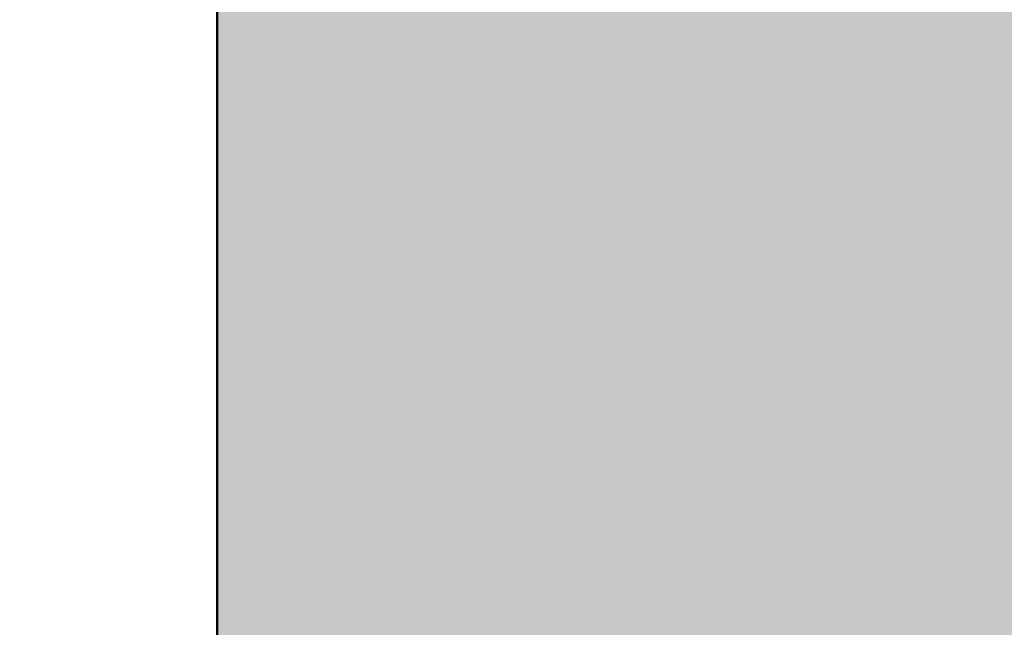
# Model space of a CAD drawing. Units: millimetres. Extents: x 0 to 2267, y 0 to 1823.
# Tile 32 of 256: x 1593.3409 to 1593.7801, y 1226.1145 to 1226.3857. Entities that reach past the tile are written whole.
import ezdxf

# ---------------------------------------------------------------- set-up
doc = ezdxf.new("R2010")
doc.units = ezdxf.units.MM
doc.header["$MEASUREMENT"] = 0
doc.layers.add('M-HATC', color=252, linetype='Continuous', lineweight=18)
doc.layers.add('M-OUTL', color=7, linetype='Continuous', lineweight=50)

msp = doc.modelspace()

# ---------------------------------------------------------------- hatches: boundary and pattern name
at = {"layer": 'M-HATC'}
h = msp.add_hatch(color=256, dxfattribs=at)
h.dxf.hatch_style = 1
h.paths.add_polyline_path([(2055.77105, 1603.06204), (1381.08677, 1603.06204), (1381.08677, 1598.06204), (2055.77105, 1598.06204)])
h.paths.add_polyline_path([(2055.77105, 1598.06204), (1381.08677, 1598.06204), (1381.08677, 1593.06204), (2055.77105, 1593.06204)])
h.paths.add_polyline_path([(2051.30737, 1536.76088), (1385.55044, 1536.76088), (1385.55044, 1526.76088), (1387.55044, 1526.76088), (1388.53662, 1525.05276), (1385.33187, 1521.23348), (1385.33187, 1521.22256), (2050.25417, 1522.74913), (2048.32119, 1525.05276), (2049.30737, 1526.76088), (2051.30737, 1526.76088)])
edge = h.paths.add_edge_path()
edge.add_arc((1847.53451, 1379.14917), 135, 222.6030607, 222.8908505, ccw=False)
edge.add_line((1748.16629, 1287.76561), (1683.09212, 1287.76561))
edge.add_arc((1583.7239, 1379.14917), 135, 317.1091495, 317.3969393, ccw=False)
edge.add_arc((1678.9686, 1290.67067), 5, 222.89085, 317.10915, ccw=False)
edge.add_arc((1774.21331, 1379.14917), 135, 222.6030607, 222.8908505, ccw=False)
edge.add_line((1674.84509, 1287.76561), (1609.77092, 1287.76561))
edge.add_arc((1510.4027, 1379.14917), 135, 317.1091495, 317.3969393, ccw=False)
edge.add_arc((1605.6474, 1290.67067), 5, 222.89085, 317.10915, ccw=False)
edge.add_arc((1700.89211, 1379.14917), 135, 222.6030607, 222.8908505, ccw=False)
edge.add_line((1601.52388, 1287.76561), (1536.44972, 1287.76561))
edge.add_arc((1437.08149, 1379.14917), 135, 317.1091495, 317.3969393, ccw=False)
edge.add_arc((1532.3262, 1290.67067), 5, 222.89085, 317.10915, ccw=False)
edge.add_arc((1627.57091, 1379.14917), 135, 222.6030607, 222.8908505, ccw=False)
edge.add_line((1528.20268, 1287.76561), (1505.92891, 1287.76561))
edge.add_spline(control_points=[(1505.92891, 1287.76561), (1504.26224, 1287.76561), (1504.26224, 1282.76561), (1505.92891, 1282.76561)], knot_values=[0, 0, 0, 0, 5, 5, 5, 5], degree=3, periodic=0)
edge.add_line((1505.92891, 1282.76561), (1930.92891, 1282.76561))
edge.add_spline(control_points=[(1930.92891, 1282.76561), (1932.59557, 1282.76561), (1932.59557, 1287.76561), (1930.92891, 1287.76561)], knot_values=[0, 0, 0, 0, 5, 5, 5, 5], degree=3, periodic=0)
edge.add_line((1930.92891, 1287.76561), (1903.05573, 1287.76561))
edge.add_arc((1803.6875, 1379.14917), 135, 317.1091495, 317.3969393, ccw=False)
edge.add_arc((1898.93221, 1290.67067), 5, 222.89085, 317.10915, ccw=False)
edge.add_arc((1994.17691, 1379.14917), 135, 222.6030607, 222.8908505, ccw=False)
edge.add_line((1894.80869, 1287.76561), (1829.73452, 1287.76561))
edge.add_arc((1730.3663, 1379.14917), 135, 317.1091495, 317.3969393, ccw=False)
edge.add_arc((1825.61101, 1290.67067), 5, 222.89085, 317.10915, ccw=False)
edge.add_arc((1920.85571, 1379.14917), 135, 222.6030607, 222.8908505, ccw=False)
edge.add_line((1821.48749, 1287.76561), (1756.41332, 1287.76561))
edge.add_arc((1657.0451, 1379.14917), 135, 317.1091495, 317.3969393, ccw=False)
edge.add_arc((1752.28981, 1290.67067), 5, 222.89085, 317.10915, ccw=False)
edge = h.paths.add_edge_path()
edge.add_spline(control_points=[(1843.42891, 1227.24746), (1845.09557, 1227.24746), (1845.09557, 1232.24746), (1843.42891, 1232.24746)], knot_values=[0, 0, 0, 0, 5, 5, 5, 5], degree=3, periodic=0)
edge.add_line((1843.42891, 1232.24746), (1593.42891, 1232.24746))
edge.add_spline(control_points=[(1593.42891, 1232.24746), (1591.76224, 1232.24746), (1591.76224, 1227.24746), (1593.42891, 1227.24746)], knot_values=[0, 0, 0, 0, 5, 5, 5, 5], degree=3, periodic=0)
edge.add_line((1593.42891, 1227.24746), (1843.42891, 1227.24746))
h.paths.add_polyline_path([(1905.92891, 1127.41706), (1530.92891, 1127.41706, 0.414214), (1520.92891, 1117.41706), (1530.92891, 1117.41706), (1915.92891, 1117.41706, 0.414214)])
edge = h.paths.add_edge_path()
edge.add_arc((1397.08577, 1498.40775), 12.72993, 90.782146, 190.878706, ccw=False)
edge.add_line((1396.912, 1511.13649), (1428.00968, 1511.34875))
edge.add_line((1428.00968, 1511.34875), (1433.00968, 1511.34875))
edge.add_line((1433.00968, 1511.34875), (1434.439, 1511.34875))
edge.add_arc((1419.474, 1498.08041), 20, 41.560995, 74.082109)
edge.add_line((1424.95919, 1517.31353), (1399.93509, 1517.25608))
edge.add_spline(control_points=[(1399.93074, 1517.25607), (1399.88398, 1517.21312), (1399.8328, 1517.16893), (1399.77741, 1517.1236)], knot_values=[11.567499, 11.567499, 11.567499, 11.567499, 11.814249, 11.814249, 11.814249, 11.814249], degree=3, periodic=0)
edge.add_spline(control_points=[(1399.63279, 1517.00986), (1399.58305, 1516.97214), (1399.53072, 1516.93375), (1399.47591, 1516.89474)], knot_values=[11.167718, 11.167718, 11.167718, 11.167718, 11.365188, 11.365188, 11.365188, 11.365188], degree=3, periodic=0)
edge.add_spline(control_points=[(1399.33981, 1516.80007), (1399.15144, 1516.67185), (1398.93836, 1516.5377), (1398.70404, 1516.39942)], knot_values=[10.376405, 10.376405, 10.376405, 10.376405, 11.00994, 11.00994, 11.00994, 11.00994], degree=3, periodic=0)
edge.add_spline(control_points=[(1398.65716, 1516.37187), (1398.57885, 1516.32602), (1398.49825, 1516.27974), (1398.41549, 1516.23309)], knot_values=[10.125175, 10.125175, 10.125175, 10.125175, 10.334406, 10.334406, 10.334406, 10.334406], degree=3, periodic=0)
edge.add_spline(control_points=[(1398.26422, 1516.14874), (1398.19595, 1516.11107), (1398.12634, 1516.07319), (1398.05546, 1516.03513)], knot_values=[9.832246, 9.832246, 9.832246, 9.832246, 9.999658, 9.999658, 9.999658, 9.999658], degree=3, periodic=0)
edge.add_spline(control_points=[(1397.9987, 1516.00476), (1397.73115, 1515.86211), (1397.44602, 1515.71707), (1397.14664, 1515.57138)], knot_values=[9.161808, 9.161808, 9.161808, 9.161808, 9.787769, 9.787769, 9.787769, 9.787769], degree=3, periodic=0)
edge.add_spline(control_points=[(1397.14664, 1515.57138), (1396.84182, 1515.42305), (1396.52223, 1515.27404), (1396.1914, 1515.12621)], knot_values=[8.524455, 8.524455, 8.524455, 8.524455, 9.161808, 9.161808, 9.161808, 9.161808], degree=3, periodic=0)
edge.add_spline(control_points=[(1396.07771, 1515.07565), (1395.98538, 1515.03478), (1395.89222, 1514.99402), (1395.7983, 1514.9534)], knot_values=[8.275193, 8.275193, 8.275193, 8.275193, 8.451726, 8.451726, 8.451726, 8.451726], degree=3, periodic=0)
edge.add_spline(control_points=[(1395.60184, 1514.86912), (1395.49975, 1514.82568), (1395.39685, 1514.78244), (1395.29322, 1514.73944)], knot_values=[7.962917, 7.962917, 7.962917, 7.962917, 8.152764, 8.152764, 8.152764, 8.152764], degree=3, periodic=0)
edge.add_spline(control_points=[(1395.21158, 1514.70568), (1394.82779, 1514.5475), (1394.43452, 1514.39287), (1394.03645, 1514.24422)], knot_values=[7.21254, 7.21254, 7.21254, 7.21254, 7.913148, 7.913148, 7.913148, 7.913148], degree=3, periodic=0)
edge.add_spline(control_points=[(1394.03645, 1514.24422), (1393.70758, 1514.12142), (1393.37544, 1514.0027), (1393.04267, 1513.88945)], knot_values=[6.633733, 6.633733, 6.633733, 6.633733, 7.21254, 7.21254, 7.21254, 7.21254], degree=3, periodic=0)
edge.add_spline(control_points=[(1392.82142, 1513.81499), (1392.71978, 1513.78118), (1392.61815, 1513.74791), (1392.51658, 1513.71521)], knot_values=[6.328796, 6.328796, 6.328796, 6.328796, 6.505493, 6.505493, 6.505493, 6.505493], degree=3, periodic=0)
edge.add_spline(control_points=[(1392.51658, 1513.71521), (1392.31873, 1513.65151), (1392.12116, 1513.59001), (1391.92441, 1513.53098)], knot_values=[5.984605, 5.984605, 5.984605, 5.984605, 6.328796, 6.328796, 6.328796, 6.328796], degree=3, periodic=0)
edge.add_spline(control_points=[(1391.79155, 1513.49146), (1391.31215, 1513.35011), (1390.83842, 1513.22392), (1390.37844, 1513.11711)], knot_values=[5.066697, 5.066697, 5.066697, 5.066697, 5.907055, 5.907055, 5.907055, 5.907055], degree=3, periodic=0)
edge.add_spline(control_points=[(1390.37844, 1513.11711), (1390.17973, 1513.07097), (1389.98359, 1513.02845), (1389.79067, 1512.98988)], knot_values=[4.70367, 4.70367, 4.70367, 4.70367, 5.066695, 5.066695, 5.066695, 5.066695], degree=3, periodic=0)
edge.add_spline(control_points=[(1389.42203, 1512.92036), (1389.24588, 1512.88922), (1389.0729, 1512.86172), (1388.90364, 1512.83814)], knot_values=[4.130571, 4.130571, 4.130571, 4.130571, 4.469816, 4.469816, 4.469816, 4.469816], degree=3, periodic=0)
edge.add_spline(control_points=[(1388.90364, 1512.83814), (1388.59103, 1512.7946), (1388.29108, 1512.76444), (1388.00714, 1512.74941)], knot_values=[3.504031, 3.504031, 3.504031, 3.504031, 4.130571, 4.130571, 4.130571, 4.130571], degree=3, periodic=0)
edge.add_spline(control_points=[(1387.9356, 1512.74593), (1387.85378, 1512.74231), (1387.77334, 1512.73997), (1387.69435, 1512.73898)], knot_values=[3.268866, 3.268866, 3.268866, 3.268866, 3.451164, 3.451164, 3.451164, 3.451164], degree=3, periodic=0)
edge.add_spline(control_points=[(1387.33512, 1512.74426), (1387.20757, 1512.74991), (1387.08472, 1512.7597), (1386.96699, 1512.77385)], knot_values=[2.670686, 2.670686, 2.670686, 2.670686, 2.984, 2.984, 2.984, 2.984], degree=3, periodic=0)
edge.add_spline(control_points=[(1386.83274, 1512.79225), (1386.82093, 1512.79407), (1386.80917, 1512.79594), (1386.79747, 1512.79787)], knot_values=[2.516981, 2.516981, 2.516981, 2.516981, 2.549528, 2.549528, 2.549528, 2.549528], degree=3, periodic=0)
edge.add_spline(control_points=[(1386.45257, 1512.87348), (1386.42573, 1512.88105), (1386.39931, 1512.88895), (1386.3733, 1512.89719)], knot_values=[2.095869, 2.095869, 2.095869, 2.095869, 2.17941, 2.17941, 2.17941, 2.17941], degree=3, periodic=0)
edge.add_spline(control_points=[(1386.06911, 1513.01889), (1386.06338, 1513.02174), (1386.05768, 1513.02463), (1386.05201, 1513.02753)], knot_values=[1.72453, 1.72453, 1.72453, 1.72453, 1.745933, 1.745933, 1.745933, 1.745933], degree=3, periodic=0)
edge.add_arc((1399.474, 1498.08041), 20, 131.824322, 180)
edge.add_arc((1630.33362, 1505.54843), 250.97076, 181.7051759, 236.427975)
edge.add_arc((1605.33992, 1483.30441), 218.7822, 238.660829, 243.3496099)
edge.add_arc((1647.09105, 1510.35917), 262.89859, 183.1298361, 237.8534422, ccw=False)
h.paths.add_polyline_path([(1406.53685, 1391.96444, 0.149382), (1491.55061, 1296.44177, -0.129517)], flags=17)
edge = h.paths.add_edge_path()
edge.add_arc((2037.38381, 1498.08041), 20, 0, 48.265868)
edge.add_spline(control_points=[(2050.69731, 1513.00525), (2050.65121, 1512.98471), (2050.60338, 1512.96554), (2050.55388, 1512.94771)], knot_values=[1.835652, 1.835652, 1.835652, 1.835652, 2.000781, 2.000781, 2.000781, 2.000781], degree=3, periodic=0)
edge.add_spline(control_points=[(2050.46156, 1512.91661), (2050.479, 1512.9221), (2050.49625, 1512.92774), (2050.51332, 1512.93353)], knot_values=[2.045477, 2.045477, 2.045477, 2.045477, 2.101389, 2.101389, 2.101389, 2.101389], degree=3, periodic=0)
edge.add_spline(control_points=[(2050.12896, 1512.83416), (2050.19843, 1512.84734), (2050.26573, 1512.86233), (2050.33075, 1512.87919)], knot_values=[2.237629, 2.237629, 2.237629, 2.237629, 2.435841, 2.435841, 2.435841, 2.435841], degree=3, periodic=0)
edge.add_spline(control_points=[(2050.09463, 1512.82783), (2050.10613, 1512.82989), (2050.11757, 1512.832), (2050.12896, 1512.83416)], knot_values=[2.435841, 2.435841, 2.435841, 2.435841, 2.468321, 2.468321, 2.468321, 2.468321], degree=3, periodic=0)
edge.add_spline(control_points=[(2049.78433, 1512.78511), (2049.85521, 1512.79219), (2049.92435, 1512.80077), (2049.99166, 1512.81088)], knot_values=[2.563852, 2.563852, 2.563852, 2.563852, 2.748541, 2.748541, 2.748541, 2.748541], degree=3, periodic=0)
edge.add_spline(control_points=[(2049.4052, 1512.76169), (2049.5364, 1512.76526), (2049.66292, 1512.77299), (2049.78433, 1512.78511)], knot_values=[2.748541, 2.748541, 2.748541, 2.748541, 3.064882, 3.064882, 3.064882, 3.064882], degree=3, periodic=0)
edge.add_spline(control_points=[(2049.16976, 1512.75968), (2049.23364, 1512.7591), (2049.29654, 1512.7594), (2049.35844, 1512.7606)], knot_values=[3.102309, 3.102309, 3.102309, 3.102309, 3.2503, 3.2503, 3.2503, 3.2503], degree=3, periodic=0)
edge.add_spline(control_points=[(2048.85727, 1512.76911), (2048.96378, 1512.76378), (2049.068, 1512.76061), (2049.16976, 1512.75968)], knot_values=[3.2503, 3.2503, 3.2503, 3.2503, 3.486069, 3.486069, 3.486069, 3.486069], degree=3, periodic=0)
edge.add_spline(control_points=[(2048.69241, 1512.77892), (2048.3729, 1512.80093), (2048.0345, 1512.84106), (2047.68175, 1512.89697)], knot_values=[3.606429, 3.606429, 3.606429, 3.606429, 4.2989, 4.2989, 4.2989, 4.2989], degree=3, periodic=0)
edge.add_spline(control_points=[(2047.68175, 1512.89697), (2047.5458, 1512.91852), (2047.40772, 1512.94241), (2047.26776, 1512.96851)], knot_values=[4.2989, 4.2989, 4.2989, 4.2989, 4.565769, 4.565769, 4.565769, 4.565769], degree=3, periodic=0)
edge.add_spline(control_points=[(2047.26776, 1512.96851), (2047.14494, 1512.99141), (2047.02067, 1513.01601), (2046.89514, 1513.04223)], knot_values=[4.565769, 4.565769, 4.565769, 4.565769, 4.799971, 4.799971, 4.799971, 4.799971], degree=3, periodic=0)
edge.add_spline(control_points=[(2046.89514, 1513.04223), (2046.52865, 1513.11875), (2046.15135, 1513.20899), (2045.7676, 1513.31068)], knot_values=[4.799971, 4.799971, 4.799971, 4.799971, 5.483718, 5.483718, 5.483718, 5.483718], degree=3, periodic=0)
edge.add_spline(control_points=[(2045.7676, 1513.31068), (2045.3724, 1513.41539), (2044.97036, 1513.53225), (2044.56625, 1513.65876)], knot_values=[5.483718, 5.483718, 5.483718, 5.483718, 6.187866, 6.187866, 6.187866, 6.187866], degree=3, periodic=0)
edge.add_spline(control_points=[(2044.56625, 1513.65876), (2044.41491, 1513.70614), (2044.26329, 1513.75487), (2044.11163, 1513.80482)], knot_values=[6.187866, 6.187866, 6.187866, 6.187866, 6.451551, 6.451551, 6.451551, 6.451551], degree=3, periodic=0)
edge.add_spline(control_points=[(2044.11163, 1513.80482), (2043.99666, 1513.84269), (2043.88167, 1513.88126), (2043.76676, 1513.92048)], knot_values=[6.451551, 6.451551, 6.451551, 6.451551, 6.651434, 6.651434, 6.651434, 6.651434], degree=3, periodic=0)
edge.add_spline(control_points=[(2043.76676, 1513.92048), (2043.37157, 1514.05536), (2042.97738, 1514.19789), (2042.58863, 1514.34575)], knot_values=[6.651434, 6.651434, 6.651434, 6.651434, 7.338879, 7.338879, 7.338879, 7.338879], degree=3, periodic=0)
edge.add_spline(control_points=[(2042.58863, 1514.34575), (2042.16431, 1514.50715), (2041.74647, 1514.67491), (2041.34086, 1514.84603)], knot_values=[7.338879, 7.338879, 7.338879, 7.338879, 8.089209, 8.089209, 8.089209, 8.089209], degree=3, periodic=0)
edge.add_spline(control_points=[(2041.34086, 1514.84603), (2041.1028, 1514.94647), (2040.86896, 1515.04806), (2040.64049, 1515.1502)], knot_values=[8.089209, 8.089209, 8.089209, 8.089209, 8.529587, 8.529587, 8.529587, 8.529587], degree=3, periodic=0)
edge.add_spline(control_points=[(2040.50999, 1515.20887), (2040.08238, 1515.40218), (2039.67475, 1515.59705), (2039.29495, 1515.78939)], knot_values=[8.613818, 8.613818, 8.613818, 8.613818, 9.44571, 9.44571, 9.44571, 9.44571], degree=3, periodic=0)
edge.add_spline(control_points=[(2039.29495, 1515.78939), (2039.0618, 1515.90746), (2038.83914, 1516.02458), (2038.62878, 1516.1398)], knot_values=[9.44571, 9.44571, 9.44571, 9.44571, 9.956404, 9.956404, 9.956404, 9.956404], degree=3, periodic=0)
edge.add_spline(control_points=[(2038.62878, 1516.1398), (2038.51874, 1516.20007), (2038.41207, 1516.25982), (2038.30903, 1516.31891)], knot_values=[9.956404, 9.956404, 9.956404, 9.956404, 10.223542, 10.223542, 10.223542, 10.223542], degree=3, periodic=0)
edge.add_spline(control_points=[(2038.30903, 1516.31891), (2038.21377, 1516.37354), (2038.12161, 1516.42762), (2038.03275, 1516.48102)], knot_values=[10.223542, 10.223542, 10.223542, 10.223542, 10.47051, 10.47051, 10.47051, 10.47051], degree=3, periodic=0)
edge.add_spline(control_points=[(2038.03275, 1516.48102), (2037.78552, 1516.62961), (2037.56388, 1516.77304), (2037.37225, 1516.909)], knot_values=[10.47051, 10.47051, 10.47051, 10.47051, 11.15767, 11.15767, 11.15767, 11.15767], degree=3, periodic=0)
edge.add_spline(control_points=[(2037.37225, 1516.909), (2037.27893, 1516.9752), (2037.19274, 1517.03963), (2037.11417, 1517.10203)], knot_values=[11.15767, 11.15767, 11.15767, 11.15767, 11.49227, 11.49227, 11.49227, 11.49227], degree=3, periodic=0)
edge.add_spline(control_points=[(2036.85638, 1517.32585), (2036.91481, 1517.26923), (2036.98143, 1517.21027), (2037.05573, 1517.14922)], knot_values=[11.577341, 11.577341, 11.577341, 11.577341, 11.91035, 11.91035, 11.91035, 11.91035], degree=3, periodic=0)
edge.add_spline(control_points=[(2036.80739, 1517.37475), (2036.82301, 1517.35865), (2036.83935, 1517.34235), (2036.85638, 1517.32585)], knot_values=[11.91035, 11.91035, 11.91035, 11.91035, 12.007402, 12.007402, 12.007402, 12.007402], degree=3, periodic=0)
edge.add_spline(control_points=[(2036.70167, 1517.494), (2036.71042, 1517.48299), (2036.71958, 1517.47185), (2036.72913, 1517.4606)], knot_values=[12.184155, 12.184155, 12.184155, 12.184155, 12.255409, 12.255409, 12.255409, 12.255409], degree=3, periodic=0)
edge.add_spline(control_points=[(2036.6159, 1517.6205), (2036.61998, 1517.61304), (2036.6243, 1517.6055), (2036.62885, 1517.59789)], knot_values=[12.487913, 12.487913, 12.487913, 12.487913, 12.541035, 12.541035, 12.541035, 12.541035], degree=3, periodic=0)
edge.add_spline(control_points=[(2036.56349, 1517.78599), (2036.56372, 1517.77936), (2036.56423, 1517.77264), (2036.56502, 1517.76582)], knot_values=[12.911761, 12.911761, 12.911761, 12.911761, 12.968286, 12.968286, 12.968286, 12.968286], degree=3, periodic=0)
edge.add_spline(control_points=[(2036.61663, 1517.93042), (2036.61248, 1517.92586), (2036.60857, 1517.92121), (2036.60491, 1517.91648)], knot_values=[13.382527, 13.382527, 13.382527, 13.382527, 13.433791, 13.433791, 13.433791, 13.433791], degree=3, periodic=0)
edge.add_spline(control_points=[(2036.74902, 1518.01695), (2036.73613, 1518.0116), (2036.72393, 1518.00601), (2036.71242, 1518.00018)], knot_values=[13.726299, 13.726299, 13.726299, 13.726299, 13.809928, 13.809928, 13.809928, 13.809928], degree=3, periodic=0)
edge.add_spline(control_points=[(2036.86043, 1518.05285), (2036.83863, 1518.04743), (2036.81809, 1518.04156), (2036.79879, 1518.03526)], knot_values=[13.910887, 13.910887, 13.910887, 13.910887, 14.02153, 14.02153, 14.02153, 14.02153], degree=3, periodic=0)
edge.add_line((2036.96387, 1518.08041), (2032.38381, 1518.08041))
edge.add_line((2032.38381, 1518.08041), (2027.38381, 1518.08041))
edge.add_line((2027.38381, 1518.08041), (2022.38381, 1518.08041))
edge.add_line((2022.38381, 1518.08041), (2017.38381, 1518.08041))
edge.add_arc((2017.38381, 1498.08041), 20, 90, 138.439005)
edge.add_line((2002.41881, 1511.34875), (2003.84813, 1511.34875))
edge.add_line((2003.84813, 1511.34875), (2008.84813, 1511.34875))
edge.add_line((2008.84813, 1511.34875), (2039.77204, 1511.13768))
edge.add_arc((2039.77204, 1498.40775), 12.72993, -10.878706, 90, ccw=False)
edge.add_arc((1789.76676, 1510.35917), 262.89859, 302.1465578, 356.8701639, ccw=False)
edge.add_arc((1831.51789, 1483.30441), 218.7822, 296.6503901, 301.339171)
edge.add_arc((1806.52419, 1505.54843), 250.97076, 303.572025, 358.2948241)
h.paths.add_polyline_path([(2030.32096, 1391.96444, -0.129517), (1945.3072, 1296.44177, 0.149382)], flags=17)
edge = h.paths.add_edge_path()
edge.add_spline(control_points=[(2037.2464, 1518.08209), (2037.28977, 1518.08098), (2037.33555, 1518.08041), (2037.3838, 1518.08041)], knot_values=[0.000012, 0.000012, 0.000012, 0.000012, 0.144754, 0.144754, 0.144754, 0.144754], degree=3, periodic=0)
edge.add_line((2037.33571, 1518.08041), (2037.00963, 1518.08041))
edge.add_spline(control_points=[(2037.00963, 1518.08041), (2036.98217, 1518.07678), (2036.95605, 1518.07266), (2036.93124, 1518.06808)], knot_values=[14.13465, 14.13465, 14.13465, 14.13465, 14.247197, 14.247197, 14.247197, 14.247197], degree=3, periodic=0)
edge.add_spline(control_points=[(2036.93124, 1518.06808), (2036.92764, 1518.06741), (2036.92407, 1518.06674), (2036.92053, 1518.06605)], knot_values=[14.118315, 14.118315, 14.118315, 14.118315, 14.13465, 14.13465, 14.13465, 14.13465], degree=3, periodic=0)
edge.add_spline(control_points=[(2036.92053, 1518.06605), (2036.9118, 1518.06436), (2036.90323, 1518.06262), (2036.89484, 1518.06081)], knot_values=[14.078086, 14.078086, 14.078086, 14.078086, 14.118315, 14.118315, 14.118315, 14.118315], degree=3, periodic=0)
edge.add_spline(control_points=[(2036.89484, 1518.06081), (2036.88304, 1518.05827), (2036.87157, 1518.05562), (2036.86043, 1518.05285)], knot_values=[14.02153, 14.02153, 14.02153, 14.02153, 14.078086, 14.078086, 14.078086, 14.078086], degree=3, periodic=0)
edge.add_spline(control_points=[(2036.86043, 1518.05285), (2036.83863, 1518.04743), (2036.81809, 1518.04156), (2036.79879, 1518.03526)], knot_values=[13.910887, 13.910887, 13.910887, 13.910887, 14.02153, 14.02153, 14.02153, 14.02153], degree=3, periodic=0)
edge.add_spline(control_points=[(2036.79879, 1518.03526), (2036.79809, 1518.03504), (2036.7974, 1518.03481), (2036.79671, 1518.03458)], knot_values=[13.906906, 13.906906, 13.906906, 13.906906, 13.910887, 13.910887, 13.910887, 13.910887], degree=3, periodic=0)
edge.add_spline(control_points=[(2036.79671, 1518.03458), (2036.78819, 1518.03178), (2036.77991, 1518.02888), (2036.77187, 1518.02591)], knot_values=[13.857826, 13.857826, 13.857826, 13.857826, 13.906906, 13.906906, 13.906906, 13.906906], degree=3, periodic=0)
edge.add_spline(control_points=[(2036.77187, 1518.02591), (2036.76402, 1518.023), (2036.75641, 1518.02002), (2036.74902, 1518.01695)], knot_values=[13.809928, 13.809928, 13.809928, 13.809928, 13.857826, 13.857826, 13.857826, 13.857826], degree=3, periodic=0)
edge.add_spline(control_points=[(2036.74902, 1518.01695), (2036.73613, 1518.0116), (2036.72393, 1518.00601), (2036.71242, 1518.00018)], knot_values=[13.726299, 13.726299, 13.726299, 13.726299, 13.809928, 13.809928, 13.809928, 13.809928], degree=3, periodic=0)
edge.add_spline(control_points=[(2036.71242, 1518.00018), (2036.71211, 1518.00002), (2036.71179, 1517.99986), (2036.71147, 1517.99969)], knot_values=[13.723993, 13.723993, 13.723993, 13.723993, 13.726299, 13.726299, 13.726299, 13.726299], degree=3, periodic=0)
edge.add_spline(control_points=[(2036.71147, 1517.99969), (2036.70634, 1517.99708), (2036.70134, 1517.99441), (2036.69648, 1517.9917)], knot_values=[13.686536, 13.686536, 13.686536, 13.686536, 13.723993, 13.723993, 13.723993, 13.723993], degree=3, periodic=0)
edge.add_spline(control_points=[(2036.69648, 1517.9917), (2036.6919, 1517.98914), (2036.68744, 1517.98654), (2036.6831, 1517.9839)], knot_values=[13.651251, 13.651251, 13.651251, 13.651251, 13.686536, 13.686536, 13.686536, 13.686536], degree=3, periodic=0)
edge.add_spline(control_points=[(2036.6831, 1517.9839), (2036.67641, 1517.97983), (2036.67001, 1517.97566), (2036.6639, 1517.97139)], knot_values=[13.596804, 13.596804, 13.596804, 13.596804, 13.651251, 13.651251, 13.651251, 13.651251], degree=3, periodic=0)
edge.add_spline(control_points=[(2036.6639, 1517.97139), (2036.66358, 1517.97117), (2036.66326, 1517.97094), (2036.66294, 1517.97072)], knot_values=[13.593956, 13.593956, 13.593956, 13.593956, 13.596804, 13.596804, 13.596804, 13.596804], degree=3, periodic=0)
edge.add_spline(control_points=[(2036.66294, 1517.97072), (2036.6603, 1517.96886), (2036.65771, 1517.96698), (2036.65518, 1517.96509)], knot_values=[13.570322, 13.570322, 13.570322, 13.570322, 13.593956, 13.593956, 13.593956, 13.593956], degree=3, periodic=0)
edge.add_spline(control_points=[(2036.65518, 1517.96509), (2036.65251, 1517.9631), (2036.64991, 1517.96108), (2036.64737, 1517.95905)], knot_values=[13.545477, 13.545477, 13.545477, 13.545477, 13.570322, 13.570322, 13.570322, 13.570322], degree=3, periodic=0)
edge.add_spline(control_points=[(2036.64737, 1517.95905), (2036.64721, 1517.95892), (2036.64705, 1517.9588), (2036.64689, 1517.95867)], knot_values=[13.543931, 13.543931, 13.543931, 13.543931, 13.545477, 13.545477, 13.545477, 13.545477], degree=3, periodic=0)
edge.add_spline(control_points=[(2036.64689, 1517.95867), (2036.64121, 1517.95411), (2036.63582, 1517.94945), (2036.63073, 1517.94468)], knot_values=[13.488237, 13.488237, 13.488237, 13.488237, 13.543931, 13.543931, 13.543931, 13.543931], degree=3, periodic=0)
edge.add_spline(control_points=[(2036.63073, 1517.94468), (2036.62817, 1517.94229), (2036.62569, 1517.93988), (2036.62329, 1517.93744)], knot_values=[13.460307, 13.460307, 13.460307, 13.460307, 13.488237, 13.488237, 13.488237, 13.488237], degree=3, periodic=0)
edge.add_spline(control_points=[(2036.62329, 1517.93744), (2036.62151, 1517.93564), (2036.61978, 1517.93383), (2036.61809, 1517.932)], knot_values=[13.439712, 13.439712, 13.439712, 13.439712, 13.460307, 13.460307, 13.460307, 13.460307], degree=3, periodic=0)
edge.add_spline(control_points=[(2036.61809, 1517.932), (2036.6176, 1517.93147), (2036.61711, 1517.93095), (2036.61663, 1517.93042)], knot_values=[13.433791, 13.433791, 13.433791, 13.433791, 13.439712, 13.439712, 13.439712, 13.439712], degree=3, periodic=0)
edge.add_spline(control_points=[(2036.61663, 1517.93042), (2036.61248, 1517.92586), (2036.60857, 1517.92121), (2036.60491, 1517.91648)], knot_values=[13.382527, 13.382527, 13.382527, 13.382527, 13.433791, 13.433791, 13.433791, 13.433791], degree=3, periodic=0)
edge.add_spline(control_points=[(2036.60491, 1517.91648), (2036.60258, 1517.91347), (2036.60036, 1517.91044), (2036.59824, 1517.90737)], knot_values=[13.350017, 13.350017, 13.350017, 13.350017, 13.382527, 13.382527, 13.382527, 13.382527], degree=3, periodic=0)
edge.add_spline(control_points=[(2036.59824, 1517.90737), (2036.59718, 1517.90585), (2036.59616, 1517.90433), (2036.59515, 1517.90279)], knot_values=[13.333922, 13.333922, 13.333922, 13.333922, 13.350017, 13.350017, 13.350017, 13.350017], degree=3, periodic=0)
edge.add_spline(control_points=[(2036.59515, 1517.90279), (2036.59452, 1517.90183), (2036.5939, 1517.90086), (2036.59329, 1517.89989)], knot_values=[13.323828, 13.323828, 13.323828, 13.323828, 13.333922, 13.333922, 13.333922, 13.333922], degree=3, periodic=0)
edge.add_spline(control_points=[(2036.59329, 1517.89989), (2036.59049, 1517.89545), (2036.5879, 1517.89094), (2036.5855, 1517.88637)], knot_values=[13.277545, 13.277545, 13.277545, 13.277545, 13.323828, 13.323828, 13.323828, 13.323828], degree=3, periodic=0)
edge.add_spline(control_points=[(2036.5855, 1517.88637), (2036.58355, 1517.88267), (2036.58174, 1517.87892), (2036.58006, 1517.87513)], knot_values=[13.240119, 13.240119, 13.240119, 13.240119, 13.277545, 13.277545, 13.277545, 13.277545], degree=3, periodic=0)
edge.add_spline(control_points=[(2036.58006, 1517.87513), (2036.57952, 1517.87393), (2036.579, 1517.87272), (2036.57849, 1517.87151)], knot_values=[13.228211, 13.228211, 13.228211, 13.228211, 13.240119, 13.240119, 13.240119, 13.240119], degree=3, periodic=0)
edge.add_spline(control_points=[(2036.57849, 1517.87151), (2036.57796, 1517.87023), (2036.57744, 1517.86896), (2036.57693, 1517.86767)], knot_values=[13.215717, 13.215717, 13.215717, 13.215717, 13.228211, 13.228211, 13.228211, 13.228211], degree=3, periodic=0)
edge.add_spline(control_points=[(2036.57693, 1517.86767), (2036.57548, 1517.86399), (2036.57414, 1517.86027), (2036.57293, 1517.85651)], knot_values=[13.179847, 13.179847, 13.179847, 13.179847, 13.215717, 13.215717, 13.215717, 13.215717], degree=3, periodic=0)
edge.add_spline(control_points=[(2036.57293, 1517.85651), (2036.5713, 1517.8515), (2036.56989, 1517.84641), (2036.56868, 1517.84126)], knot_values=[13.132017, 13.132017, 13.132017, 13.132017, 13.179847, 13.179847, 13.179847, 13.179847], degree=3, periodic=0)
edge.add_spline(control_points=[(2036.56868, 1517.84126), (2036.56844, 1517.84023), (2036.56821, 1517.8392), (2036.56798, 1517.83817)], knot_values=[13.122482, 13.122482, 13.122482, 13.122482, 13.132017, 13.132017, 13.132017, 13.132017], degree=3, periodic=0)
edge.add_spline(control_points=[(2036.56798, 1517.83817), (2036.56758, 1517.83634), (2036.56721, 1517.8345), (2036.56687, 1517.83266)], knot_values=[13.105592, 13.105592, 13.105592, 13.105592, 13.122482, 13.122482, 13.122482, 13.122482], degree=3, periodic=0)
edge.add_spline(control_points=[(2036.56687, 1517.83266), (2036.56622, 1517.82921), (2036.56567, 1517.82574), (2036.5652, 1517.82223)], knot_values=[13.074063, 13.074063, 13.074063, 13.074063, 13.105592, 13.105592, 13.105592, 13.105592], degree=3, periodic=0)
edge.add_spline(control_points=[(2036.5652, 1517.82223), (2036.5652, 1517.82223), (2036.5652, 1517.82223), (2036.5652, 1517.82223)], knot_values=[13.074043, 13.074043, 13.074043, 13.074043, 13.074063, 13.074063, 13.074063, 13.074063], degree=3, periodic=0)
edge.add_spline(control_points=[(2036.5652, 1517.82223), (2036.56443, 1517.81643), (2036.5639, 1517.81055), (2036.56361, 1517.8046)], knot_values=[13.021884, 13.021884, 13.021884, 13.021884, 13.074043, 13.074043, 13.074043, 13.074043], degree=3, periodic=0)
edge.add_spline(control_points=[(2036.56361, 1517.8046), (2036.56358, 1517.80401), (2036.56356, 1517.80342), (2036.56353, 1517.80283)], knot_values=[13.01674, 13.01674, 13.01674, 13.01674, 13.021884, 13.021884, 13.021884, 13.021884], degree=3, periodic=0)
edge.add_spline(control_points=[(2036.56353, 1517.80283), (2036.56344, 1517.80051), (2036.56338, 1517.79817), (2036.56336, 1517.79582)], knot_values=[12.996438, 12.996438, 12.996438, 12.996438, 13.01674, 13.01674, 13.01674, 13.01674], degree=3, periodic=0)
edge.add_spline(control_points=[(2036.56336, 1517.79582), (2036.56334, 1517.79257), (2036.56338, 1517.78929), (2036.56349, 1517.78599)], knot_values=[12.968286, 12.968286, 12.968286, 12.968286, 12.996438, 12.996438, 12.996438, 12.996438], degree=3, periodic=0)
edge.add_spline(control_points=[(2036.56349, 1517.78599), (2036.56372, 1517.77936), (2036.56423, 1517.77264), (2036.56502, 1517.76582)], knot_values=[12.911761, 12.911761, 12.911761, 12.911761, 12.968286, 12.968286, 12.968286, 12.968286], degree=3, periodic=0)
edge.add_spline(control_points=[(2036.56502, 1517.76582), (2036.56503, 1517.76573), (2036.56504, 1517.76564), (2036.56505, 1517.76555)], knot_values=[12.911017, 12.911017, 12.911017, 12.911017, 12.911761, 12.911761, 12.911761, 12.911761], degree=3, periodic=0)
edge.add_spline(control_points=[(2036.56505, 1517.76555), (2036.56541, 1517.76245), (2036.56583, 1517.75933), (2036.56631, 1517.75619)], knot_values=[12.88528, 12.88528, 12.88528, 12.88528, 12.911017, 12.911017, 12.911017, 12.911017], degree=3, periodic=0)
edge.add_spline(control_points=[(2036.56631, 1517.75619), (2036.56673, 1517.75341), (2036.5672, 1517.75062), (2036.56771, 1517.74782)], knot_values=[12.862519, 12.862519, 12.862519, 12.862519, 12.88528, 12.88528, 12.88528, 12.88528], degree=3, periodic=0)
edge.add_spline(control_points=[(2036.56771, 1517.74782), (2036.56779, 1517.74737), (2036.56788, 1517.74692), (2036.56796, 1517.74647)], knot_values=[12.858885, 12.858885, 12.858885, 12.858885, 12.862519, 12.862519, 12.862519, 12.862519], degree=3, periodic=0)
edge.add_spline(control_points=[(2036.56796, 1517.74647), (2036.5692, 1517.73986), (2036.57069, 1517.73316), (2036.57243, 1517.72638)], knot_values=[12.8053, 12.8053, 12.8053, 12.8053, 12.858885, 12.858885, 12.858885, 12.858885], degree=3, periodic=0)
edge.add_spline(control_points=[(2036.57243, 1517.72638), (2036.5734, 1517.72257), (2036.57446, 1517.71874), (2036.57559, 1517.71488)], knot_values=[12.775176, 12.775176, 12.775176, 12.775176, 12.8053, 12.8053, 12.8053, 12.8053], degree=3, periodic=0)
edge.add_spline(control_points=[(2036.57559, 1517.71488), (2036.57628, 1517.71252), (2036.577, 1517.71015), (2036.57775, 1517.70778)], knot_values=[12.756759, 12.756759, 12.756759, 12.756759, 12.775176, 12.775176, 12.775176, 12.775176], degree=3, periodic=0)
edge.add_spline(control_points=[(2036.57775, 1517.70778), (2036.57808, 1517.70674), (2036.57841, 1517.7057), (2036.57875, 1517.70466)], knot_values=[12.748742, 12.748742, 12.748742, 12.748742, 12.756759, 12.756759, 12.756759, 12.756759], degree=3, periodic=0)
edge.add_spline(control_points=[(2036.57875, 1517.70466), (2036.58082, 1517.6983), (2036.58309, 1517.69187), (2036.58557, 1517.68537)], knot_values=[12.69959, 12.69959, 12.69959, 12.69959, 12.748742, 12.748742, 12.748742, 12.748742], degree=3, periodic=0)
edge.add_spline(control_points=[(2036.58557, 1517.68537), (2036.58762, 1517.68001), (2036.5898, 1517.6746), (2036.59213, 1517.66916)], knot_values=[12.659038, 12.659038, 12.659038, 12.659038, 12.69959, 12.69959, 12.69959, 12.69959], degree=3, periodic=0)
edge.add_spline(control_points=[(2036.59213, 1517.66916), (2036.59397, 1517.66482), (2036.59591, 1517.66047), (2036.59793, 1517.65608)], knot_values=[12.626806, 12.626806, 12.626806, 12.626806, 12.659038, 12.659038, 12.659038, 12.659038], degree=3, periodic=0)
edge.add_spline(control_points=[(2036.59793, 1517.65608), (2036.59839, 1517.65507), (2036.59886, 1517.65406), (2036.59934, 1517.65305)], knot_values=[12.619394, 12.619394, 12.619394, 12.619394, 12.626806, 12.626806, 12.626806, 12.626806], degree=3, periodic=0)
edge.add_spline(control_points=[(2036.59934, 1517.65305), (2036.60435, 1517.64236), (2036.60987, 1517.63151), (2036.61589, 1517.6205)], knot_values=[12.541039, 12.541039, 12.541039, 12.541039, 12.619394, 12.619394, 12.619394, 12.619394], degree=3, periodic=0)
edge.add_spline(control_points=[(2036.61589, 1517.6205), (2036.61589, 1517.6205), (2036.6159, 1517.6205), (2036.6159, 1517.6205)], knot_values=[12.541035, 12.541035, 12.541035, 12.541035, 12.541039, 12.541039, 12.541039, 12.541039], degree=3, periodic=0)
edge.add_spline(control_points=[(2036.6159, 1517.6205), (2036.61998, 1517.61304), (2036.6243, 1517.6055), (2036.62885, 1517.59789)], knot_values=[12.487913, 12.487913, 12.487913, 12.487913, 12.541035, 12.541035, 12.541035, 12.541035], degree=3, periodic=0)
edge.add_spline(control_points=[(2036.62885, 1517.59789), (2036.63261, 1517.5916), (2036.63653, 1517.58526), (2036.64061, 1517.57888)], knot_values=[12.443982, 12.443982, 12.443982, 12.443982, 12.487913, 12.487913, 12.487913, 12.487913], degree=3, periodic=0)
edge.add_spline(control_points=[(2036.64061, 1517.57888), (2036.64144, 1517.57757), (2036.64228, 1517.57626), (2036.64313, 1517.57495)], knot_values=[12.434996, 12.434996, 12.434996, 12.434996, 12.443982, 12.443982, 12.443982, 12.443982], degree=3, periodic=0)
edge.add_spline(control_points=[(2036.64313, 1517.57495), (2036.65306, 1517.55958), (2036.66389, 1517.54394), (2036.6756, 1517.52803)], knot_values=[12.329647, 12.329647, 12.329647, 12.329647, 12.434996, 12.434996, 12.434996, 12.434996], degree=3, periodic=0)
edge.add_spline(control_points=[(2036.6756, 1517.52803), (2036.68385, 1517.51682), (2036.69254, 1517.50548), (2036.70167, 1517.494)], knot_values=[12.255409, 12.255409, 12.255409, 12.255409, 12.329647, 12.329647, 12.329647, 12.329647], degree=3, periodic=0)
edge.add_spline(control_points=[(2036.70167, 1517.494), (2036.71042, 1517.48299), (2036.71958, 1517.47185), (2036.72913, 1517.4606)], knot_values=[12.184155, 12.184155, 12.184155, 12.184155, 12.255409, 12.255409, 12.255409, 12.255409], degree=3, periodic=0)
edge.add_spline(control_points=[(2036.72913, 1517.4606), (2036.74363, 1517.44352), (2036.75904, 1517.42617), (2036.77534, 1517.40855)], knot_values=[12.075961, 12.075961, 12.075961, 12.075961, 12.184155, 12.184155, 12.184155, 12.184155], degree=3, periodic=0)
edge.add_spline(control_points=[(2036.77534, 1517.40855), (2036.77631, 1517.4075), (2036.77729, 1517.40645), (2036.77827, 1517.40539)], knot_values=[12.069502, 12.069502, 12.069502, 12.069502, 12.075961, 12.075961, 12.075961, 12.075961], degree=3, periodic=0)
edge.add_spline(control_points=[(2036.77827, 1517.40539), (2036.78768, 1517.39526), (2036.79739, 1517.38505), (2036.80739, 1517.37475)], knot_values=[12.007402, 12.007402, 12.007402, 12.007402, 12.069502, 12.069502, 12.069502, 12.069502], degree=3, periodic=0)
edge.add_spline(control_points=[(2036.80739, 1517.37475), (2036.82301, 1517.35865), (2036.83935, 1517.34235), (2036.85638, 1517.32585)], knot_values=[11.91035, 11.91035, 11.91035, 11.91035, 12.007402, 12.007402, 12.007402, 12.007402], degree=3, periodic=0)
edge.add_spline(control_points=[(2036.85638, 1517.32585), (2036.91481, 1517.26923), (2036.98143, 1517.21027), (2037.05573, 1517.14922)], knot_values=[11.577341, 11.577341, 11.577341, 11.577341, 11.91035, 11.91035, 11.91035, 11.91035], degree=3, periodic=0)
edge.add_spline(control_points=[(2037.05573, 1517.14922), (2037.07471, 1517.13362), (2037.0942, 1517.11789), (2037.11417, 1517.10203)], knot_values=[11.49227, 11.49227, 11.49227, 11.49227, 11.577341, 11.577341, 11.577341, 11.577341], degree=3, periodic=0)
edge.add_spline(control_points=[(2037.11417, 1517.10203), (2037.19274, 1517.03963), (2037.27893, 1516.9752), (2037.37225, 1516.909)], knot_values=[11.15767, 11.15767, 11.15767, 11.15767, 11.49227, 11.49227, 11.49227, 11.49227], degree=3, periodic=0)
edge.add_spline(control_points=[(2037.37225, 1516.909), (2037.56388, 1516.77304), (2037.78552, 1516.62961), (2038.03275, 1516.48102)], knot_values=[10.47051, 10.47051, 10.47051, 10.47051, 11.15767, 11.15767, 11.15767, 11.15767], degree=3, periodic=0)
edge.add_spline(control_points=[(2038.03275, 1516.48102), (2038.12161, 1516.42762), (2038.21377, 1516.37354), (2038.30903, 1516.31891)], knot_values=[10.223542, 10.223542, 10.223542, 10.223542, 10.47051, 10.47051, 10.47051, 10.47051], degree=3, periodic=0)
edge.add_spline(control_points=[(2038.30903, 1516.31891), (2038.41207, 1516.25982), (2038.51874, 1516.20007), (2038.62878, 1516.1398)], knot_values=[9.956404, 9.956404, 9.956404, 9.956404, 10.223542, 10.223542, 10.223542, 10.223542], degree=3, periodic=0)
edge.add_spline(control_points=[(2038.62878, 1516.1398), (2038.83914, 1516.02458), (2039.0618, 1515.90746), (2039.29495, 1515.78939)], knot_values=[9.44571, 9.44571, 9.44571, 9.44571, 9.956404, 9.956404, 9.956404, 9.956404], degree=3, periodic=0)
edge.add_spline(control_points=[(2039.29495, 1515.78939), (2039.67475, 1515.59705), (2040.08238, 1515.40218), (2040.50999, 1515.20887)], knot_values=[8.613818, 8.613818, 8.613818, 8.613818, 9.44571, 9.44571, 9.44571, 9.44571], degree=3, periodic=0)
edge.add_spline(control_points=[(2040.50999, 1515.20887), (2040.55329, 1515.1893), (2040.59679, 1515.16974), (2040.64049, 1515.1502)], knot_values=[8.529587, 8.529587, 8.529587, 8.529587, 8.613818, 8.613818, 8.613818, 8.613818], degree=3, periodic=0)
edge.add_spline(control_points=[(2040.64049, 1515.1502), (2040.86896, 1515.04806), (2041.1028, 1514.94647), (2041.34086, 1514.84603)], knot_values=[8.089209, 8.089209, 8.089209, 8.089209, 8.529587, 8.529587, 8.529587, 8.529587], degree=3, periodic=0)
edge.add_spline(control_points=[(2041.34086, 1514.84603), (2041.74647, 1514.67491), (2042.16431, 1514.50715), (2042.58863, 1514.34575)], knot_values=[7.338879, 7.338879, 7.338879, 7.338879, 8.089209, 8.089209, 8.089209, 8.089209], degree=3, periodic=0)
edge.add_spline(control_points=[(2042.58863, 1514.34575), (2042.97738, 1514.19789), (2043.37157, 1514.05536), (2043.76676, 1513.92048)], knot_values=[6.651434, 6.651434, 6.651434, 6.651434, 7.338879, 7.338879, 7.338879, 7.338879], degree=3, periodic=0)
edge.add_spline(control_points=[(2043.76676, 1513.92048), (2043.88167, 1513.88126), (2043.99666, 1513.84269), (2044.11163, 1513.80482)], knot_values=[6.451551, 6.451551, 6.451551, 6.451551, 6.651434, 6.651434, 6.651434, 6.651434], degree=3, periodic=0)
edge.add_spline(control_points=[(2044.11163, 1513.80482), (2044.26329, 1513.75487), (2044.41491, 1513.70614), (2044.56625, 1513.65876)], knot_values=[6.187866, 6.187866, 6.187866, 6.187866, 6.451551, 6.451551, 6.451551, 6.451551], degree=3, periodic=0)
edge.add_spline(control_points=[(2044.56625, 1513.65876), (2044.97036, 1513.53225), (2045.3724, 1513.41539), (2045.7676, 1513.31068)], knot_values=[5.483718, 5.483718, 5.483718, 5.483718, 6.187866, 6.187866, 6.187866, 6.187866], degree=3, periodic=0)
edge.add_spline(control_points=[(2045.7676, 1513.31068), (2046.15135, 1513.20899), (2046.52865, 1513.11875), (2046.89514, 1513.04223)], knot_values=[4.799971, 4.799971, 4.799971, 4.799971, 5.483718, 5.483718, 5.483718, 5.483718], degree=3, periodic=0)
edge.add_spline(control_points=[(2046.89514, 1513.04223), (2047.02067, 1513.01601), (2047.14494, 1512.99141), (2047.26776, 1512.96851)], knot_values=[4.565769, 4.565769, 4.565769, 4.565769, 4.799971, 4.799971, 4.799971, 4.799971], degree=3, periodic=0)
edge.add_spline(control_points=[(2047.26776, 1512.96851), (2047.40772, 1512.94241), (2047.5458, 1512.91852), (2047.68175, 1512.89697)], knot_values=[4.2989, 4.2989, 4.2989, 4.2989, 4.565769, 4.565769, 4.565769, 4.565769], degree=3, periodic=0)
edge.add_spline(control_points=[(2047.68175, 1512.89697), (2048.0345, 1512.84106), (2048.3729, 1512.80093), (2048.69241, 1512.77892)], knot_values=[3.606429, 3.606429, 3.606429, 3.606429, 4.2989, 4.2989, 4.2989, 4.2989], degree=3, periodic=0)
edge.add_spline(control_points=[(2048.69241, 1512.77892), (2048.74794, 1512.7751), (2048.8029, 1512.77182), (2048.85727, 1512.76911)], knot_values=[3.486069, 3.486069, 3.486069, 3.486069, 3.606429, 3.606429, 3.606429, 3.606429], degree=3, periodic=0)
edge.add_spline(control_points=[(2048.85727, 1512.76911), (2048.96378, 1512.76378), (2049.068, 1512.76061), (2049.16976, 1512.75968)], knot_values=[3.2503, 3.2503, 3.2503, 3.2503, 3.486069, 3.486069, 3.486069, 3.486069], degree=3, periodic=0)
edge.add_spline(control_points=[(2049.16976, 1512.75968), (2049.23364, 1512.7591), (2049.29654, 1512.7594), (2049.35844, 1512.7606)], knot_values=[3.102309, 3.102309, 3.102309, 3.102309, 3.2503, 3.2503, 3.2503, 3.2503], degree=3, periodic=0)
edge.add_spline(control_points=[(2049.35844, 1512.7606), (2049.37409, 1512.76091), (2049.38968, 1512.76127), (2049.4052, 1512.76169)], knot_values=[3.064882, 3.064882, 3.064882, 3.064882, 3.102309, 3.102309, 3.102309, 3.102309], degree=3, periodic=0)
edge.add_spline(control_points=[(2049.4052, 1512.76169), (2049.5364, 1512.76526), (2049.66292, 1512.77299), (2049.78433, 1512.78511)], knot_values=[2.748541, 2.748541, 2.748541, 2.748541, 3.064882, 3.064882, 3.064882, 3.064882], degree=3, periodic=0)
edge.add_spline(control_points=[(2049.78433, 1512.78511), (2049.85521, 1512.79219), (2049.92435, 1512.80077), (2049.99166, 1512.81088)], knot_values=[2.563852, 2.563852, 2.563852, 2.563852, 2.748541, 2.748541, 2.748541, 2.748541], degree=3, periodic=0)
edge.add_spline(control_points=[(2049.99166, 1512.81088), (2050.02648, 1512.81612), (2050.0608, 1512.82177), (2050.09463, 1512.82783)], knot_values=[2.468321, 2.468321, 2.468321, 2.468321, 2.563852, 2.563852, 2.563852, 2.563852], degree=3, periodic=0)
edge.add_spline(control_points=[(2050.09463, 1512.82783), (2050.10613, 1512.82989), (2050.11757, 1512.832), (2050.12896, 1512.83416)], knot_values=[2.435841, 2.435841, 2.435841, 2.435841, 2.468321, 2.468321, 2.468321, 2.468321], degree=3, periodic=0)
edge.add_spline(control_points=[(2050.12896, 1512.83416), (2050.19843, 1512.84734), (2050.26573, 1512.86233), (2050.33075, 1512.87919)], knot_values=[2.237629, 2.237629, 2.237629, 2.237629, 2.435841, 2.435841, 2.435841, 2.435841], degree=3, periodic=0)
edge.add_spline(control_points=[(2050.33075, 1512.87919), (2050.37544, 1512.89077), (2050.41906, 1512.90324), (2050.46156, 1512.91661)], knot_values=[2.101389, 2.101389, 2.101389, 2.101389, 2.237629, 2.237629, 2.237629, 2.237629], degree=3, periodic=0)
edge.add_spline(control_points=[(2050.46156, 1512.91661), (2050.479, 1512.9221), (2050.49625, 1512.92774), (2050.51332, 1512.93353)], knot_values=[2.045477, 2.045477, 2.045477, 2.045477, 2.101389, 2.101389, 2.101389, 2.101389], degree=3, periodic=0)
edge.add_spline(control_points=[(2050.51332, 1512.93353), (2050.52696, 1512.93816), (2050.54048, 1512.94288), (2050.55388, 1512.94771)], knot_values=[2.000781, 2.000781, 2.000781, 2.000781, 2.045477, 2.045477, 2.045477, 2.045477], degree=3, periodic=0)
edge.add_spline(control_points=[(2050.55388, 1512.94771), (2050.60338, 1512.96554), (2050.65121, 1512.98471), (2050.69731, 1513.00525)], knot_values=[1.835652, 1.835652, 1.835652, 1.835652, 2.000781, 2.000781, 2.000781, 2.000781], degree=3, periodic=0)
edge.add_arc((2037.38381, 1498.08041), 20, 48.265868, 90.129934)
edge = h.paths.add_edge_path(flags=16)
edge.add_spline(control_points=[(1386.13885, 1512.98591), (1388.91997, 1511.73946), (1398.03873, 1515.51866), (1399.93074, 1517.25607)], knot_values=[1.831046, 1.831046, 1.831046, 1.831046, 11.814249, 11.814249, 11.814249, 11.814249], degree=3, periodic=0)
edge.add_line((1399.93074, 1517.25607), (1393.74348, 1517.24186))
edge.add_arc((1399.474, 1498.08041), 20, 106.650105, 131.817301)
h = msp.add_hatch(color=256, dxfattribs=at)
h.dxf.hatch_style = 1
h.paths.add_polyline_path([(2042.88863, 1580.17963), (2055.77105, 1593.06204), (1381.08677, 1593.06204), (1393.96918, 1580.17963), (1374.08597, 1560.29642), (2062.77184, 1560.29642)])
h.paths.add_polyline_path([(1843.42891, 1201.32971), (1843.42891, 1227.24746), (1593.42891, 1227.24746), (1593.42891, 1201.32971, -0.228274), (1574.59893, 1162.23457), (1530.92891, 1127.41706), (1905.92891, 1127.41706), (1862.25888, 1162.23457, -0.228274)])

# ---------------------------------------------------------------- linework, layer by layer
at = {"layer": 'M-OUTL'}
msp.add_line((1593.42891, 1201.32971), (1593.42891, 1227.24746), dxfattribs=at)

doc.saveas('drawing.dxf')
